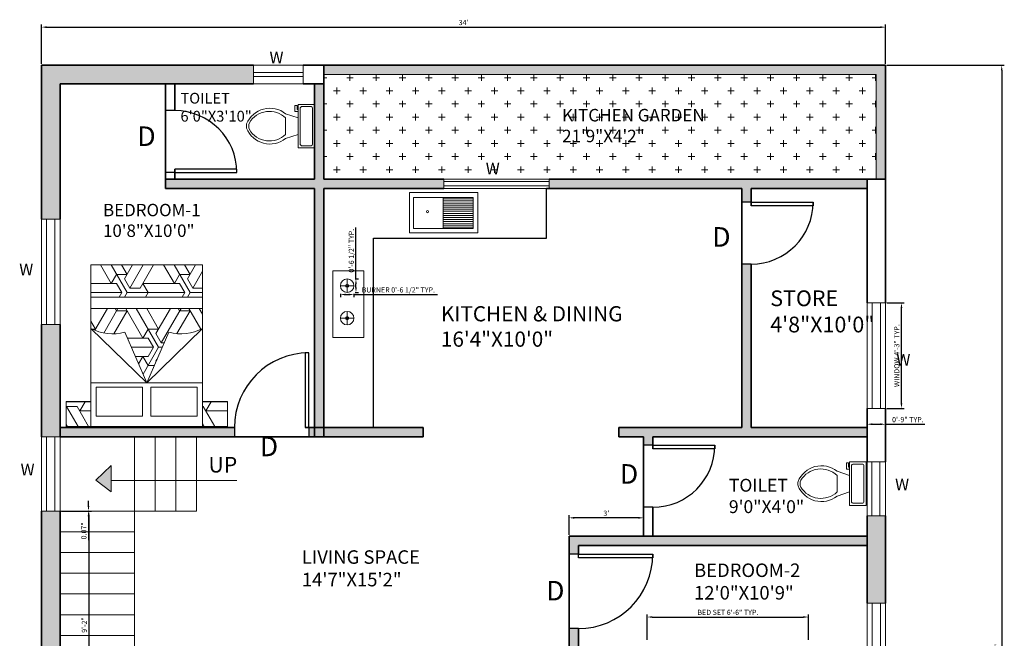
# Model space of a CAD drawing. Units: inches. Extents: x 1878 to 2382, y 1889 to 2524.
# Tile 2 of 2: x 1906 to 2382, y 2225 to 2524. Entities that reach past the tile are written whole.
import ezdxf

# ---------------------------------------------------------------- set-up
doc = ezdxf.new("R2010")
doc.units = ezdxf.units.IN
for name, color, linetype, lineweight in [('A-ANNO-DIMS', 2, 'Continuous', 18), ('A-ANNO-SYMB', 7, 'Continuous', 18), ('A-ANNO-TEXT', 7, 'Continuous', 18), ('A-AREA-IDEN', 7, 'Continuous', 18), ('A-DOOR', 4, 'Continuous', 25), ('A-EQPM', 8, 'Continuous', 18), ('A-FLOR-CASE', 8, 'Continuous', 25), ('A-FLOR-FIXT', 8, 'Continuous', 18), ('A-FLOR-FIXT-PATT', 8, 'Continuous', 13), ('A-FLOR-STRS', 7, 'Continuous', 18), ('A-FURN', 8, 'Continuous', 18), ('A-FURN-PATT', 252, 'Continuous', 13), ('A-WALL', 7, 'Continuous', 35), ('A-WALL-PATT', 251, 'Continuous', 13), ('L-PLNT', 3, 'Continuous', 18), ('L-PLNT-PATT', 3, 'Continuous', 13), ('windows', 5, 'Continuous', 18)]:
    doc.layers.add(name, color=color, linetype=linetype, lineweight=lineweight)
doc.styles.get("Standard").update_dxf_attribs({"font": 'arial.ttf'})
doc.dimstyles.new('ISO-25', dxfattribs={"dimtxt": 2.5, "dimasz": 2.5, "dimexe": 1.25, "dimexo": 0.625, "dimtad": 1, "dimlunit": 3, "dimtxsty": 'Standard', "dimcen": 2.5, "dimadec": 0, "dimazin": 0, "dimtfac": 1, "dimtmove": 0, "dimatfit": 3, "dimfxl": 1, "dimarcsym": 0})

# ---------------------------------------------------------------- blocks, each defined once
blk = doc.blocks.new('*U2')
for p, q in [((0, 0), (0, -4)), ((36, 0), (36, -4))]:
    blk.add_line(p, q)
blk.add_lwpolyline([(0, 0), (0, 36), (1.75, 36), (1.75, 0)], close=True)
blk.add_arc((0, 0), 36, 0, 90)
blk = doc.blocks.new('*U4')
for p, q in [((0, 0), (0, -4)), ((30, 0), (30, -4))]:
    blk.add_line(p, q)
blk.add_lwpolyline([(0, 0), (0, 30), (1.75, 30), (1.75, 0)], close=True)
blk.add_arc((0, 0), 30, 0, 90)
blk = doc.blocks.new('*U3')
for p, q in [((0, 0), (0, -4)), ((30, 0), (30, -4))]:
    blk.add_line(p, q)
blk.add_lwpolyline([(0, 0), (0, 30), (1.75, 30), (1.75, 0)], close=True)
blk.add_arc((0, 0), 30, 0, 90)
blk = doc.blocks.new('*U5')
for p, q in [((-30, 0), (-30, -4)), ((0, 0), (0, -4))]:
    blk.add_line(p, q)
blk.add_lwpolyline([(0, 0), (0, 30), (-1.75, 30), (-1.75, 0)], close=True)
blk.add_arc((0, 0), 30, 90, 180)
blk = doc.blocks.new('*U6')
for p, q in [((0, 0), (0, -4)), ((-36, 0), (-36, -4))]:
    blk.add_line(p, q)
blk.add_lwpolyline([(0, 0), (0, 36), (-1.75, 36), (-1.75, 0)], close=True)
blk.add_arc((0, 0), 36, 90, 180)
blk = doc.blocks.new('*U8')
for p, q in [((9.5, -6), (9.5, -2)), ((-10, -8.5), (-8, -8.5)), ((-10, -9.5), (-10, -8.5)), ((-7, -9.5), (-10, -9.5)), ((-8, -8.5), (-8, -8)), ((-7, -8), (-7, -9.5)), ((-4, -8), (-6, -14)), ((4, -8), (6, -14)), ((4, -14), (-4, -14))]:
    blk.add_line(p, q)
blk.add_lwpolyline([(10.5, -8), (10.5, 0), (-10.5, 0), (-10.5, -8)], close=True)
for points in [[(-9.5, -2), (-9.5, -6)], [(8.5, -1), (-8.5, -1)], [(-8.5, -7), (8.5, -7)]]:
    blk.add_lwpolyline(points)
for centre, radius, start, end in [((-8.62, -1.88), 0.884, 81.8699, 188.1301), ((8.62, -1.88), 0.884, 351.8699, 98.1301), ((-8.62, -6.12), 0.884, 171.8699, 278.1301), ((8.62, -6.12), 0.884, 261.8699, 8.1301), ((3.52, -21.58), 12.17, 141.4691, 247.9714), ((4.2, -21.82), 11.33, 136.3677, 238.9468), ((-3.52, -21.58), 12.17, 292.0284, 38.5307), ((-4.2, -21.82), 11.33, 301.053, 43.6321), ((0, -27.88), 4, 245.7318, 294.2682), ((0, -29), 4, 254.8605, 285.1395)]:
    blk.add_arc(centre, radius, start, end)
blk = doc.blocks.new('*D9')
at = {"layer": 'A-ANNO-DIMS', "color": 0, "lineweight": -2, "transparency": 16777216}
for p, q in [((1925.87, 2286.07), (1940.42, 2286.07)), ((1939.17, 2283.57), (1939.17, 2178.57)), ((1925.87, 2176.07), (1940.42, 2176.07))]:
    blk.add_line(p, q, dxfattribs=at)
at = {"layer": 'A-ANNO-DIMS', "color": 0, "transparency": 16777216}
for points in [[(1938.75, 2283.57), (1939.59, 2283.57), (1939.17, 2286.07)], [(1938.75, 2178.57), (1939.59, 2178.57), (1939.17, 2176.07)]]:
    blk.add_solid(points, dxfattribs=at)
at = {"layer": 'Defpoints', "color": 0, "transparency": 16777216}
for p in [(1925.24, 2286.07), (1925.24, 2176.07), (1939.17, 2176.07)]:
    blk.add_point(p, dxfattribs=at)
at = {"layer": 'A-ANNO-DIMS', "color": 0, "transparency": 16777216, "insert": (1937.27, 2231.07), "char_height": 2.5, "attachment_point": 5, "rotation": 90}
blk.add_mtext('9\'-2"', dxfattribs=at)
blk = doc.blocks.new('*D10')
at = {"layer": 'A-ANNO-DIMS', "color": 0, "lineweight": -2, "transparency": 16777216}
for p, q in [((1938.96, 2288.64), (1938.96, 2291.14)), ((1925.87, 2286.14), (1940.21, 2286.14)), ((1925.87, 2286.07), (1940.21, 2286.07)), ((1938.96, 2286.14), (1938.96, 2286.07)), ((1938.96, 2283.57), (1938.96, 2272.09))]:
    blk.add_line(p, q, dxfattribs=at)
at = {"layer": 'A-ANNO-DIMS', "color": 0, "transparency": 16777216}
for points in [[(1938.55, 2288.64), (1939.38, 2288.64), (1938.96, 2286.14)], [(1938.55, 2283.57), (1939.38, 2283.57), (1938.96, 2286.07)]]:
    blk.add_solid(points, dxfattribs=at)
at = {"layer": 'Defpoints', "color": 0, "transparency": 16777216}
for p in [(1925.24, 2286.14), (1925.24, 2286.07), (1938.96, 2286.07)]:
    blk.add_point(p, dxfattribs=at)
at = {"layer": 'A-ANNO-DIMS', "color": 0, "transparency": 16777216, "insert": (1937.06, 2276.58), "char_height": 2.5, "attachment_point": 5, "rotation": 90}
blk.add_mtext('0.07"', dxfattribs=at)
blk = doc.blocks.new('*D13')
at = {"layer": 'A-ANNO-DIMS', "color": 0, "lineweight": -2, "transparency": 16777216}
for p, q in [((2171.24, 2274.69), (2171.24, 2284.12)), ((2204.74, 2282.87), (2173.74, 2282.87)), ((2207.24, 2274.69), (2207.24, 2284.12))]:
    blk.add_line(p, q, dxfattribs=at)
at = {"layer": 'A-ANNO-DIMS', "color": 0, "transparency": 16777216}
for points in [[(2173.74, 2283.29), (2173.74, 2282.45), (2171.24, 2282.87)], [(2204.74, 2283.29), (2204.74, 2282.45), (2207.24, 2282.87)]]:
    blk.add_solid(points, dxfattribs=at)
at = {"layer": 'Defpoints', "color": 0, "transparency": 16777216}
for p in [(2171.24, 2282.87), (2171.24, 2274.07), (2207.24, 2274.07)]:
    blk.add_point(p, dxfattribs=at)
at = {"layer": 'A-ANNO-DIMS', "color": 0, "transparency": 16777216, "insert": (2189.24, 2284.77), "char_height": 2.5, "attachment_point": 5}
blk.add_mtext("3'", dxfattribs=at)
blk = doc.blocks.new('*D14')
at = {"layer": 'A-ANNO-DIMS', "color": 0, "lineweight": -2, "transparency": 16777216}
for p, q in [((1916.24, 2502.19), (1916.24, 2521.22)), ((1918.74, 2519.97), (2321.74, 2519.97)), ((2324.24, 2502.19), (2324.24, 2521.22))]:
    blk.add_line(p, q, dxfattribs=at)
at = {"layer": 'A-ANNO-DIMS', "color": 0, "transparency": 16777216}
for points in [[(1918.74, 2520.39), (1918.74, 2519.55), (1916.24, 2519.97)], [(2321.74, 2520.39), (2321.74, 2519.55), (2324.24, 2519.97)]]:
    blk.add_solid(points, dxfattribs=at)
at = {"layer": 'Defpoints', "color": 0, "transparency": 16777216}
for p in [(2324.24, 2519.97), (1916.24, 2501.57), (2324.24, 2501.57)]:
    blk.add_point(p, dxfattribs=at)
at = {"layer": 'A-ANNO-DIMS', "color": 0, "transparency": 16777216, "insert": (2120.24, 2521.87), "char_height": 2.5, "attachment_point": 5}
blk.add_mtext("34'", dxfattribs=at)
blk = doc.blocks.new('*D15')
at = {"layer": 'A-ANNO-DIMS', "color": 0, "lineweight": -2, "transparency": 16777216}
for p, q in [((2324.87, 2501.57), (2381.6, 2501.57)), ((2380.35, 2499.07), (2380.35, 1940.07)), ((2324.87, 1937.57), (2381.6, 1937.57))]:
    blk.add_line(p, q, dxfattribs=at)
at = {"layer": 'A-ANNO-DIMS', "color": 0, "transparency": 16777216}
for points in [[(2379.94, 2499.07), (2380.77, 2499.07), (2380.35, 2501.57)], [(2379.94, 1940.07), (2380.77, 1940.07), (2380.35, 1937.57)]]:
    blk.add_solid(points, dxfattribs=at)
at = {"layer": 'Defpoints', "color": 0, "transparency": 16777216}
for p in [(2324.24, 2501.57), (2324.24, 1937.57), (2380.35, 1937.57)]:
    blk.add_point(p, dxfattribs=at)
at = {"layer": 'A-ANNO-DIMS', "color": 0, "transparency": 16777216, "insert": (2378.48, 2219.57), "char_height": 2.5, "attachment_point": 5, "rotation": 90}
blk.add_mtext("47'", dxfattribs=at)
blk = doc.blocks.new('BED-DOUBLE-WITH-NIGHTSTANDS')
for p, q in [((39, 21.08), (12, 47.35)), ((39, 21.08), (28.35, 45.54)), ((39, 21.08), (66, 47.35)), ((39, 21.08), (49.65, 45.54)), ((66, 21.08), (12, 21.08)), ((36.92, 4.84), (36.92, 18.87)), ((40.92, 4.84), (40.92, 18.87)), ((0, 0), (0, 12)), ((0, 12), (12, 12)), ((78, 12), (66, 12)), ((78, 12), (78, 0)), ((12, 0), (0, 0)), ((66, 0), (78, 0))]:
    blk.add_line(p, q)
for points in [[(66, 78), (12, 78), (12, 0), (66, 0)], [(66, 56.97), (12, 56.97), (12, 62.38), (66, 62.38)]]:
    blk.add_lwpolyline(points, close=True)
for points in [[(36.92, 4.84), (14.54, 4.84), (14.54, 18.87), (36.92, 18.87)], [(40.92, 18.87), (63.29, 18.87), (63.29, 4.84), (40.92, 4.84)]]:
    blk.add_lwpolyline(points)
for centre, start, end in [((22.35, 66.17), 241.1931, 286.2111), ((55.65, 66.17), 253.7889, 298.8069)]:
    blk.add_arc(centre, 21.48, start, end)
blk = doc.blocks.new('WIN-51IN')
for p, q in [((4.5, 51), (0, 51)), ((0, 51), (9, 51)), ((0, 0), (0, 51)), ((2.5, 0), (2.5, 51)), ((6.5, 0), (6.5, 51)), ((9, 51), (9, 0)), ((0, 0), (9, 0)), ((9, 0), (4.5, 0))]:
    blk.add_line(p, q)
blk = doc.blocks.new('COOKTOP-BURNER')
for p, q in [((3.27, 6.54), (3.27, 0)), ((0, 3.27), (6.54, 3.27))]:
    blk.add_line(p, q)
for radius in [3.27, 0.76]:
    blk.add_circle((3.27, 3.27), radius)
blk = doc.blocks.new('*D21')
at = {"layer": 'A-ANNO-DIMS', "color": 0, "lineweight": -2, "transparency": 16777216}
for p, q in [((2209, 2223.87), (2209, 2236.19)), ((2211.5, 2234.94), (2284.5, 2234.94)), ((2287, 2223.87), (2287, 2236.19))]:
    blk.add_line(p, q, dxfattribs=at)
at = {"layer": 'A-ANNO-DIMS', "color": 0, "transparency": 16777216}
for points in [[(2211.5, 2235.36), (2211.5, 2234.53), (2209, 2234.94)], [(2284.5, 2235.36), (2284.5, 2234.53), (2287, 2234.94)]]:
    blk.add_solid(points, dxfattribs=at)
at = {"layer": 'Defpoints', "color": 0, "transparency": 16777216}
for p in [(2287, 2234.94), (2209, 2223.24), (2287, 2223.24)]:
    blk.add_point(p, dxfattribs=at)
at = {"layer": 'A-ANNO-DIMS', "color": 0, "transparency": 16777216, "insert": (2248, 2236.86), "char_height": 2.5, "attachment_point": 5}
blk.add_mtext('BED SET 6\'-6" TYP.', dxfattribs=at)
blk = doc.blocks.new('*D23')
at = {"layer": 'A-ANNO-DIMS', "color": 0, "lineweight": -2, "transparency": 16777216}
for p, q in [((2324.87, 2386.74), (2333.14, 2386.74)), ((2331.89, 2338.24), (2331.89, 2384.24)), ((2324.87, 2335.74), (2333.14, 2335.74))]:
    blk.add_line(p, q, dxfattribs=at)
at = {"layer": 'A-ANNO-DIMS', "color": 0, "transparency": 16777216}
for points in [[(2331.47, 2384.24), (2332.31, 2384.24), (2331.89, 2386.74)], [(2331.47, 2338.24), (2332.31, 2338.24), (2331.89, 2335.74)]]:
    blk.add_solid(points, dxfattribs=at)
at = {"layer": 'Defpoints', "color": 0, "transparency": 16777216}
for p in [(2324.24, 2386.74), (2331.89, 2386.74), (2324.24, 2335.74)]:
    blk.add_point(p, dxfattribs=at)
at = {"layer": 'A-ANNO-DIMS', "color": 0, "transparency": 16777216, "insert": (2329.97, 2361.24), "char_height": 2.5, "attachment_point": 5, "rotation": 90}
blk.add_mtext('WINDOW 4\'-3" TYP.', dxfattribs=at)
blk = doc.blocks.new('*D24')
at = {"layer": 'A-ANNO-DIMS', "color": 0, "lineweight": -2, "transparency": 16777216}
for p, q in [((2315.24, 2335.12), (2315.24, 2326.84)), ((2324.24, 2335.12), (2324.24, 2326.84)), ((2317.74, 2328.09), (2321.74, 2328.09)), ((2324.24, 2328.09), (2343.23, 2328.09))]:
    blk.add_line(p, q, dxfattribs=at)
at = {"layer": 'A-ANNO-DIMS', "color": 0, "transparency": 16777216}
for points in [[(2317.74, 2328.51), (2317.74, 2327.68), (2315.24, 2328.09)], [(2321.74, 2328.51), (2321.74, 2327.68), (2324.24, 2328.09)]]:
    blk.add_solid(points, dxfattribs=at)
at = {"layer": 'Defpoints', "color": 0, "transparency": 16777216}
for p in [(2315.24, 2335.74), (2324.24, 2335.74), (2324.24, 2328.09)]:
    blk.add_point(p, dxfattribs=at)
at = {"layer": 'A-ANNO-DIMS', "color": 0, "transparency": 16777216, "insert": (2334.99, 2330), "char_height": 2.5, "attachment_point": 5}
blk.add_mtext('0\'-9" TYP.', dxfattribs=at)
blk = doc.blocks.new('*D25')
at = {"layer": 'A-ANNO-DIMS', "color": 0, "lineweight": -2, "transparency": 16777216}
for p, q in [((2060.72, 2391.12), (2060.72, 2389.51)), ((2063.22, 2390.76), (2064.76, 2390.76)), ((2067.26, 2391.12), (2067.26, 2389.51)), ((2067.26, 2390.76), (2107.68, 2390.76))]:
    blk.add_line(p, q, dxfattribs=at)
at = {"layer": 'A-ANNO-DIMS', "color": 0, "transparency": 16777216}
for points in [[(2063.22, 2391.18), (2063.22, 2390.34), (2060.72, 2390.76)], [(2064.76, 2391.18), (2064.76, 2390.34), (2067.26, 2390.76)]]:
    blk.add_solid(points, dxfattribs=at)
at = {"layer": 'Defpoints', "color": 0, "transparency": 16777216}
for p in [(2060.72, 2391.74), (2067.26, 2391.74), (2067.26, 2390.76)]:
    blk.add_point(p, dxfattribs=at)
at = {"layer": 'A-ANNO-DIMS', "color": 0, "transparency": 16777216, "insert": (2088.72, 2392.68), "char_height": 2.5, "attachment_point": 5}
blk.add_mtext('BURNER 0\'-6 1/2" TYP.', dxfattribs=at)
blk = doc.blocks.new('*D26')
at = {"layer": 'A-ANNO-DIMS', "color": 0, "lineweight": -2, "transparency": 16777216}
for p, q in [((2068.24, 2398.28), (2068.24, 2423.09)), ((2067.88, 2398.28), (2069.49, 2398.28)), ((2068.24, 2394.24), (2068.24, 2395.78)), ((2067.88, 2391.74), (2069.49, 2391.74))]:
    blk.add_line(p, q, dxfattribs=at)
at = {"layer": 'A-ANNO-DIMS', "color": 0, "transparency": 16777216}
for points in [[(2067.82, 2395.78), (2068.66, 2395.78), (2068.24, 2398.28)], [(2067.82, 2394.24), (2068.66, 2394.24), (2068.24, 2391.74)]]:
    blk.add_solid(points, dxfattribs=at)
at = {"layer": 'Defpoints', "color": 0, "transparency": 16777216}
for p in [(2067.26, 2398.28), (2068.24, 2398.28), (2067.26, 2391.74)]:
    blk.add_point(p, dxfattribs=at)
at = {"layer": 'A-ANNO-DIMS', "color": 0, "transparency": 16777216, "insert": (2066.32, 2411.94), "char_height": 2.5, "attachment_point": 5, "rotation": 90}
blk.add_mtext('0\'-6 1/2" TYP.', dxfattribs=at)

msp = doc.modelspace()

# ---------------------------------------------------------------- hatches: boundary and pattern name
at = {"layer": 'A-ANNO-SYMB'}
h = msp.add_hatch(color=256, dxfattribs=at)
h.dxf.hatch_style = 1
h.paths.add_polyline_path([(1949.873, 2308.099), (1942.575, 2300.99), (1949.873, 2295.451)])
at = {"layer": 'A-FLOR-FIXT-PATT'}
h = msp.add_hatch(dxfattribs=at)
h.set_pattern_fill('ANSI31', color=256, scale=0.3149606, angle=-45, style=0)
h.paths.add_polyline_path([(2110.458, 2422.666), (2124.915, 2422.666), (2124.915, 2437.672), (2110.458, 2437.672)])
at = {"layer": 'A-FURN-PATT'}
h = msp.add_hatch(dxfattribs=at)
h.set_pattern_fill('ESCHER', color=256, angle=180)
h.set_pattern_definition([(240, (4365.518, 4820.139), (30.48, 7e-09), [27.94, -2.54]), (360, (4365.518, 4820.139), (-15.24, 26.39645), [27.94, -2.54]), (120, (4365.518, 4820.139), (-30.48, 7e-09), [27.94, -2.54]), (240, (4362.978, 4820.139), (30.48, 7e-09), [5.08, -25.4]), (120, (4362.978, 4820.139), (-30.48, 7e-09), [5.08, -25.4]), (240, (4366.788, 4817.94), (30.48, 7e-09), [5.08, -25.4]), (360, (4366.788, 4817.94), (-15.24, 26.39645), [5.08, -25.4]), (120, (4366.788, 4822.338), (-30.48, 7e-09), [5.08, -25.4]), (360, (4366.788, 4822.338), (-15.24, 26.39645), [5.08, -25.4]), (240, (4375.678, 4820.139), (30.48, 7e-09), [5.08, -25.4]), (120, (4375.678, 4820.139), (-30.48, 7e-09), [5.08, -25.4]), (240, (4360.438, 4828.937), (30.48, 7e-09), [5.08, -25.4]), (360, (4360.438, 4828.937), (-15.24, 26.39645), [5.08, -25.4]), (120, (4360.438, 4811.34), (-30.48, 7e-09), [5.08, -25.4]), (360, (4360.438, 4811.34), (-15.24, 26.39645), [5.08, -25.4]), (180, (4360.438, 4815.74), (15.24, -26.39645), [17.78, -12.7]), (180, (4360.438, 4824.538), (15.24, -26.39645), [17.78, -12.7]), (300, (4364.248, 4813.54), (30.48, -7e-09), [17.78, -12.7]), (300, (4371.868, 4817.94), (30.48, -7e-09), [17.78, -12.7]), (60, (4371.868, 4822.338), (-15.24, 26.39645), [17.78, -12.7]), (60, (4364.248, 4826.738), (-15.24, 26.39645), [17.78, -12.7])])
h.paths.add_polyline_path([(1967.133, 2348.159), (1977.782, 2372.62, 0.1989938), (1994.133, 2374.424), (1994.133, 2384.048), (1940.133, 2384.048), (1940.133, 2374.424, 0.1989938), (1956.484, 2372.62)])
h.paths.add_polyline_path([(1994.133, 2389.462), (1994.133, 2405.079), (1940.133, 2405.079), (1940.133, 2389.462)])
h.paths.add_polyline_path([(1928.133, 2339.079), (1928.133, 2327.079), (1940.133, 2327.079), (1940.133, 2339.079)])
h.paths.add_polyline_path([(2006.133, 2339.079), (1994.133, 2339.079), (1994.133, 2327.079), (2006.133, 2327.079)])
at = {"layer": 'A-WALL-PATT'}
h = msp.add_hatch(color=256, dxfattribs=at)
h.dxf.hatch_style = 1
h.paths.add_polyline_path([(1925.241, 2376.261), (1916.241, 2376.261), (1916.241, 2322.068), (1920.741, 2322.068), (1925.241, 2322.068)])
h.paths.add_polyline_path([(1925.241, 2286.14), (1916.241, 2286.068), (1916.241, 2097.507), (1920.741, 2097.507), (1925.241, 2097.507)])
h.paths.add_polyline_path([(1925.241, 2046.507), (1916.241, 2046.507), (1916.241, 1993.068), (1925.241, 1993.068), (2100.229, 1993.068), (2100.229, 1997.568), (2100.229, 2002.068), (2052.741, 2002.068), (2052.741, 2135.568), (2048.241, 2135.568), (2048.241, 2002.068), (1925.241, 2002.068)])
h.paths.add_polyline_path([(2175.741, 2006.935), (2175.253, 2006.935), (2171.241, 2006.935), (2171.241, 2002.068), (2136.229, 2002.068), (2136.229, 1993.068), (2171.241, 1993.068), (2175.741, 1993.068)])
h.paths.add_polyline_path([(1925.241, 2492.568), (2018.709, 2492.568), (2018.709, 2497.068), (2018.709, 2501.568), (1916.241, 2501.568), (1916.241, 2427.261), (1925.241, 2427.261)])
h.paths.add_polyline_path([(2324.241, 2501.568), (2052.741, 2501.568), (2052.741, 2497.068), (2319.741, 2497.068), (2319.741, 2446.568), (2324.241, 2446.568)])
h.paths.add_polyline_path([(2110.638, 2446.568), (2052.741, 2446.568), (2052.741, 2492.568), (2048.241, 2492.568), (2048.241, 2446.568), (1976.241, 2446.568), (1976.241, 2442.068), (2048.241, 2442.068), (2048.241, 2326.568), (2052.741, 2326.568), (2052.741, 2442.068), (2110.638, 2442.068), (2110.638, 2444.318)])
h.paths.add_polyline_path([(2100.741, 2326.568), (2052.741, 2326.568), (2052.741, 2322.068), (2100.741, 2322.068)])
h.paths.add_polyline_path([(2052.741, 2326.568), (2048.241, 2326.568), (2048.241, 2322.068), (2052.741, 2322.068)])
h.paths.add_polyline_path([(2048.241, 2326.568), (2045.469, 2326.568), (2045.469, 2326.565), (2045.469, 2322.565), (2045.469, 2322.068), (2048.241, 2322.068)])
h.paths.add_polyline_path([(2009.469, 2326.568), (1925.241, 2326.568), (1925.241, 2322.068), (2009.469, 2322.068), (2009.469, 2322.565)])
h.paths.add_polyline_path([(2315.241, 2326.568), (2259.241, 2326.568), (2259.241, 2405.456), (2255.232, 2405.456), (2254.741, 2405.456), (2254.741, 2326.568), (2207.241, 2326.568), (2195.241, 2326.568), (2195.241, 2322.068), (2207.241, 2322.068), (2207.241, 2317.983), (2207.736, 2317.983), (2211.741, 2317.983), (2211.741, 2322.068), (2315.241, 2322.068)])
h.paths.add_polyline_path([(2315.241, 2446.568), (2161.638, 2446.568), (2161.638, 2442.068), (2254.741, 2442.068), (2254.741, 2435.456), (2255.232, 2435.456), (2259.241, 2435.456), (2259.241, 2442.068), (2315.241, 2442.068)])
h.paths.add_polyline_path([(2315.241, 2274.068), (2207.241, 2274.068), (2171.241, 2274.068), (2171.241, 2265.326), (2171.731, 2265.326), (2175.741, 2265.326), (2175.741, 2269.568), (2315.241, 2269.568)])
h.paths.add_polyline_path([(2226.778, 2011.849), (2261.831, 2011.849), (2261.831, 2029.017), (2226.778, 2029.017)], flags=9)
h.paths.add_polyline_path([(2187.32, 2282.174), (2191.18, 2282.174), (2191.18, 2287.326), (2187.32, 2287.326)], flags=9)
h.paths.add_polyline_path([(2140.304, 2010.813), (2177.357, 2010.813), (2177.357, 2025.4), (2140.304, 2025.4)], flags=9)
h.paths.add_polyline_path([(2106.343, 2361.376), (2203.937, 2361.376), (2203.937, 2388.801), (2106.343, 2388.801)], flags=9)
h.paths.add_polyline_path([(2229.025, 2239.686), (2287.846, 2239.686), (2287.846, 2264.045), (2229.025, 2264.045)], flags=9)
h.paths.add_polyline_path([(2039.47, 2246.058), (2106.461, 2246.058), (2106.461, 2270.435), (2039.47, 2270.435)], flags=9)
h.paths.add_polyline_path([(2080.264, 2072.343), (2149.799, 2072.343), (2149.799, 2093.991), (2080.264, 2093.991)], flags=9)
h = msp.add_hatch(color=256, dxfattribs=at)
h.dxf.hatch_style = 1
h.paths.add_polyline_path([(2324.241, 2283.876), (2315.241, 2283.876), (2315.241, 2241.596), (2324.241, 2241.596)])
h.paths.add_polyline_path([(2324.241, 2190.596), (2315.241, 2190.596), (2315.241, 1946.568), (2315.241, 1937.568), (2324.241, 1937.568)])
h.paths.add_polyline_path([(2315.241, 2145.068), (2175.741, 2145.068), (2175.741, 2229.326), (2171.731, 2229.326), (2171.241, 2229.326), (2171.241, 2145.068), (2171.241, 2140.568), (2171.241, 2140.068), (2160.741, 2140.068), (2160.741, 2135.568), (2171.241, 2135.568), (2171.241, 2042.935), (2175.253, 2042.935), (2175.741, 2042.935), (2175.741, 2140.068), (2315.241, 2140.068)])
at = {"layer": 'L-PLNT-PATT'}
h = msp.add_hatch(dxfattribs=at)
h.set_pattern_fill('CROSS', color=256)
h.paths.add_polyline_path([(2319.741, 2497.068), (2052.741, 2497.068), (2052.741, 2492.568), (2052.741, 2446.568), (2315.241, 2446.568), (2319.741, 2446.568)])

# ---------------------------------------------------------------- linework, layer by layer
at = {"layer": 'A-ANNO-SYMB'}
for p, q in [((1949.873, 2308.099), (1942.575, 2300.99)), ((1949.873, 2295.451), (1949.873, 2308.099)), ((1942.575, 2300.99), (1949.873, 2295.451)), ((2010.617, 2300.952), (1949.873, 2300.952)), ((1949.873, 2300.952), (1949.873, 2295.451))]:
    msp.add_line(p, q, dxfattribs=at)
at = {"layer": 'A-DOOR'}
for p, q in [((1976.689, 2479.666), (1976.241, 2479.666)), ((1976.689, 2479.666), (1976.689, 2479.666)), ((1976.689, 2449.666), (1976.241, 2449.666)), ((2255.232, 2435.456), (2254.741, 2435.456)), ((2255.232, 2405.456), (2254.741, 2405.456)), ((2009.469, 2322.565), (2009.469, 2322.068)), ((2045.469, 2322.565), (2045.469, 2322.068)), ((2207.736, 2317.983), (2207.241, 2317.983)), ((2207.736, 2287.983), (2207.241, 2287.983)), ((2171.731, 2265.326), (2171.241, 2265.326)), ((2171.731, 2229.326), (2171.241, 2229.326))]:
    msp.add_line(p, q, dxfattribs=at)
at = {"layer": 'A-EQPM'}
msp.add_lwpolyline([(2057.035, 2402.205), (2072.05, 2402.205), (2072.05, 2370.086), (2057.035, 2370.086)], close=True, dxfattribs=at)
at = {"layer": 'A-FLOR-CASE'}
for p, q in [((2160.349, 2418.068), (2160.349, 2442.068)), ((2076.741, 2326.568), (2076.741, 2418.068)), ((2076.741, 2418.068), (2160.349, 2418.068))]:
    msp.add_line(p, q, dxfattribs=at)
at = {"layer": 'A-FLOR-FIXT'}
msp.add_line((2110.458, 2437.672), (2110.458, 2422.666), dxfattribs=at)
for points in [[(2094.139, 2440.028), (2127.149, 2440.028), (2127.149, 2420.558), (2094.139, 2420.558)], [(2096.001, 2437.672), (2124.915, 2437.672), (2124.915, 2422.666), (2096.001, 2422.666)]]:
    msp.add_lwpolyline(points, close=True, dxfattribs=at)
msp.add_circle((2102.839, 2430.858), 0.534, dxfattribs=at)
at = {"layer": 'A-FLOR-STRS'}
for p, q in [((1961.241, 2286.068), (1961.241, 2322.068)), ((1971.241, 2286.068), (1971.241, 2322.068)), ((1981.241, 2286.068), (1981.241, 2322.068)), ((1991.241, 2286.068), (1991.241, 2322.068)), ((1925.241, 2286.068), (1925.241, 2176.068)), ((1925.241, 2286.068), (1961.241, 2286.068)), ((1961.241, 2286.068), (1961.241, 2276.068)), ((1961.241, 2286.068), (1991.241, 2286.068)), ((1961.241, 2276.068), (1925.241, 2276.068)), ((1961.241, 2276.068), (1961.241, 2176.068)), ((1961.241, 2266.068), (1925.241, 2266.068)), ((1961.241, 2256.068), (1925.241, 2256.068)), ((1961.241, 2246.068), (1925.241, 2246.068)), ((1961.241, 2236.068), (1925.241, 2236.068)), ((1961.241, 2226.068), (1925.241, 2226.068))]:
    msp.add_line(p, q, dxfattribs=at)
at = {"layer": 'A-WALL'}
for p, q in [((1916.241, 2501.568), (2018.709, 2501.568)), ((1916.241, 2427.261), (1916.241, 2501.568)), ((2042.709, 2501.568), (2324.241, 2501.568)), ((2052.741, 2492.568), (2052.741, 2501.568)), ((2324.241, 2501.568), (2324.241, 2386.744)), ((1925.241, 2492.568), (2018.709, 2492.568)), ((1925.241, 2427.261), (1925.241, 2492.568)), ((1976.241, 2442.068), (1976.241, 2492.568)), ((1980.741, 2479.666), (1980.741, 2492.568)), ((2042.709, 2492.568), (2052.741, 2492.568)), ((2048.241, 2446.568), (2048.241, 2492.568)), ((2052.741, 2446.568), (2052.741, 2492.568)), ((1980.741, 2446.568), (1980.741, 2451.416)), ((1976.241, 2446.568), (2048.241, 2446.568)), ((2052.741, 2446.568), (2110.638, 2446.568)), ((2161.638, 2446.568), (2315.241, 2446.568)), ((2315.241, 2446.568), (2315.241, 2386.744)), ((2315.241, 2446.568), (2324.241, 2446.568)), ((1976.241, 2442.068), (2048.241, 2442.068)), ((2048.241, 2322.068), (2048.241, 2442.068)), ((2052.741, 2322.068), (2052.741, 2442.068)), ((2052.741, 2442.068), (2110.638, 2442.068)), ((2160.349, 2442.068), (2254.741, 2442.068)), ((2254.741, 2442.068), (2254.741, 2326.568)), ((2259.241, 2442.068), (2259.241, 2433.706)), ((2259.241, 2442.068), (2315.241, 2442.068)), ((2259.241, 2405.456), (2259.241, 2326.568)), ((1916.241, 2322.068), (1916.241, 2376.261)), ((1925.241, 2322.068), (1925.241, 2376.261)), ((2315.241, 2335.744), (2315.241, 2309.876)), ((2324.241, 2335.744), (2324.241, 2309.876)), ((2009.469, 2326.568), (1925.241, 2326.568)), ((2052.741, 2326.568), (2043.719, 2326.568)), ((2052.741, 2326.568), (2100.741, 2326.568)), ((2100.741, 2326.568), (2100.741, 2322.068)), ((2195.241, 2322.068), (2195.241, 2326.568)), ((2195.241, 2326.568), (2207.241, 2326.568)), ((2254.741, 2326.568), (2207.241, 2326.568)), ((2259.241, 2326.568), (2315.241, 2326.568)), ((2052.741, 2322.068), (1925.241, 2322.068)), ((2100.741, 2322.068), (2052.741, 2322.068)), ((2207.241, 2322.068), (2195.241, 2322.068)), ((2207.241, 2322.068), (2207.241, 2274.068)), ((2207.241, 2322.068), (2207.241, 2318.068)), ((2315.241, 2322.068), (2211.741, 2322.068)), ((2211.741, 2322.068), (2211.741, 2316.233)), ((2254.741, 2322.068), (2315.241, 2322.068)), ((1916.241, 2097.507), (1916.241, 2286.068)), ((1925.241, 2286.14), (1925.241, 2286.068)), ((1925.241, 2097.507), (1925.241, 2286.14)), ((2211.741, 2287.983), (2211.741, 2274.068)), ((2315.241, 2283.876), (2315.241, 2241.596)), ((2324.241, 2283.876), (2324.241, 2241.596)), ((2207.241, 2274.068), (2171.241, 2274.068)), ((2171.241, 2274.068), (2171.241, 2269.568)), ((2171.241, 2145.068), (2171.241, 2274.068)), ((2315.241, 2274.068), (2207.241, 2274.068)), ((2175.741, 2269.568), (2315.241, 2269.568)), ((2175.741, 2265.326), (2175.741, 2269.568)), ((2175.741, 2145.068), (2175.741, 2229.326))]:
    msp.add_line(p, q, dxfattribs=at)
at = {"layer": 'L-PLNT'}
for p, q in [((2052.741, 2497.068), (2319.741, 2497.068)), ((2319.741, 2497.068), (2319.741, 2446.568))]:
    msp.add_line(p, q, dxfattribs=at)
at = {"layer": 'windows'}
for p, q in [((2018.709, 2501.568), (2018.709, 2492.568)), ((2018.709, 2501.568), (2042.709, 2501.568)), ((2042.709, 2497.068), (2042.709, 2501.568)), ((2042.709, 2501.568), (2042.709, 2492.568)), ((2018.709, 2498.068), (2042.709, 2498.068)), ((2018.709, 2492.568), (2018.709, 2497.068)), ((2018.709, 2496.068), (2042.709, 2496.068)), ((2042.709, 2492.568), (2018.709, 2492.568)), ((2110.638, 2446.568), (2110.638, 2442.068)), ((2161.638, 2446.568), (2110.638, 2446.568)), ((2161.638, 2444.318), (2161.638, 2446.568)), ((2161.638, 2446.568), (2161.638, 2442.068)), ((2110.638, 2445.318), (2161.638, 2445.318)), ((2110.638, 2442.068), (2110.638, 2444.318)), ((2110.638, 2443.318), (2161.638, 2443.318)), ((2161.638, 2442.068), (2110.638, 2442.068)), ((1920.741, 2427.261), (1916.241, 2427.261)), ((1916.241, 2427.261), (1925.241, 2427.261)), ((1916.241, 2427.261), (1916.241, 2376.261)), ((1918.741, 2376.261), (1918.741, 2427.261)), ((1922.741, 2376.261), (1922.741, 2427.261)), ((1925.241, 2427.261), (1925.241, 2376.261)), ((1925.241, 2376.261), (1916.241, 2376.261)), ((1916.241, 2376.261), (1920.741, 2376.261)), ((1925.241, 2322.068), (1916.241, 2322.068)), ((1916.241, 2322.068), (1920.741, 2322.068)), ((1916.241, 2322.068), (1916.241, 2286.068)), ((1918.741, 2322.068), (1918.741, 2286.14)), ((1922.741, 2322.068), (1922.741, 2286.14)), ((1925.241, 2322.068), (1925.241, 2286.14)), ((2314.768, 2309.876), (2324.241, 2309.876)), ((2315.241, 2283.876), (2315.241, 2309.876)), ((2317.505, 2307.876), (2317.505, 2309.876)), ((2324.241, 2309.876), (2319.505, 2309.876)), ((2321.505, 2307.876), (2321.505, 2309.876)), ((2324.241, 2309.876), (2324.241, 2283.876)), ((2317.505, 2307.876), (2317.505, 2283.876)), ((2321.505, 2307.876), (2321.505, 2283.876)), ((1925.241, 2286.14), (1916.241, 2286.068)), ((1920.741, 2286.14), (1925.241, 2286.14)), ((2319.505, 2283.876), (2315.241, 2283.876)), ((2315.241, 2283.876), (2324.241, 2283.876))]:
    msp.add_line(p, q, dxfattribs=at)

# ---------------------------------------------------------------- block references
at = {"layer": 'A-DOOR', "rotation": 270}
for name, p in [('*U5', (1980.689, 2449.666)), ('*U3', (2259.232, 2435.456)), ('*U4', (2211.736, 2317.983)), ('*U2', (2175.731, 2265.326))]:
    msp.add_blockref(name, p, dxfattribs=at)
at = {"layer": 'A-DOOR'}
msp.add_blockref('*U6', (2045.469, 2326.565), dxfattribs=at)
at = {"layer": 'A-EQPM'}
for p in [(2060.72, 2391.741), (2060.72, 2376.086)]:
    msp.add_blockref('COOKTOP-BURNER', p, dxfattribs=at)
at = {"layer": 'A-FLOR-FIXT', "rotation": 270}
for p in [(2048.261, 2472.14), (2314.768, 2299.376)]:
    msp.add_blockref('*U8', p, dxfattribs=at)
at = {"layer": 'A-FURN'}
msp.add_blockref('BED-DOUBLE-WITH-NIGHTSTANDS', (1928.133, 2327.079), dxfattribs=at)
at = {"layer": 'windows'}
msp.add_blockref('WIN-51IN', (2315.241, 2335.743), dxfattribs=at)
at = {"layer": 'windows', "extrusion": (0, 0, -1), "zscale": -1}
msp.add_blockref('WIN-51IN', (-2324.242, 2190.595), dxfattribs=at)

# ---------------------------------------------------------------- texts
at = {"layer": 'A-ANNO-TEXT', "attachment_point": 1}
for s, width, gutter_width, insert, char_height in [('W', 334.92413, 28.121, (2026.461, 2508.128), 5.624), ('D', 211.86968, 47.154, (1962.573, 2471.986), 9.431), ('W', 334.92413, 28.121, (2130.986, 2454.429), 5.624), ('D', 211.86968, 47.154, (2240.441, 2423.326), 9.431), ('W', 334.92413, 28.121, (1905.51, 2405.676), 5.624), ('W', 334.92413, 28.121, (2329.457, 2362.015), 5.624), ('D', 211.86968, 47.154, (2021.777, 2322.068), 9.431), ('W', 334.92413, 28.121, (1906.154, 2309.006), 5.624), ('UP', 63.8866, 37.641, (1996.94, 2312.302), 7.5281), ('D', 211.86968, 47.154, (2195.805, 2308.802), 9.431), ('W', 334.92413, 28.121, (2328.842, 2301.797), 5.624), ('D', 211.86968, 47.154, (2160.165, 2252.385), 9.431)]:
    msp.add_mtext_dynamic_manual_height_columns(s, width=width, gutter_width=gutter_width, heights=[0], dxfattribs=dict(at, insert=insert, char_height=char_height))
at = {"layer": 'A-AREA-IDEN', "attachment_point": 1}
for s, width, gutter_width, heights, insert, char_height in [('TOILET\\P6\'0"X3\'10"', 21.36598, 26.035, [0], (1983.408, 2488.234), 5.2071), ('KITCHEN GARDEN\\P21\'9"X4\'2"', 152.24218, 30.172, [0], (2167.874, 2480.46), 6.03443), ('BEDROOM-1\\P10\'8"X10\'0"', 112.45203, 29.973, [0], (1945.995, 2434.597), 5.99464), ('STORE\\P4\'8"X10\'0"', 127.23393, 38.034, [0], (2268.481, 2392.764), 7.6067), ('KITCHEN & DINING\\P16\'4"X10\'0"', 132.28599, 36.748, [0], (2109.298, 2385.143), 7.34952), ('TOILET\\P9\'0"X4\'0"', 62.32474, 31.051, [0], (2248.482, 2301.717), 6.2102), ('LIVING SPACE \\P14\'7"X15\'2"\\P ', 67.57238, 32.665, [28.447], (2042.097, 2267.184), 6.53292), ('BEDROOM-2\\P12\'0"X10\'9" ', 128.90971, 32.641, [0], (2231.65, 2260.801), 6.52814)]:
    msp.add_mtext_dynamic_manual_height_columns(s, width=width, gutter_width=gutter_width, heights=heights, dxfattribs=dict(at, insert=insert, char_height=char_height))

# ---------------------------------------------------------------- dimensions: what is measured, and where the dimension line sits
at = {"layer": 'A-ANNO-DIMS'}
for base, p1, p2, picture, middle in [((2324.241, 2519.97), (1916.241, 2501.568), (2324.241, 2501.568), '*D14', (2120.241, 2521.872)), ((2171.241, 2282.87), (2207.241, 2274.068), (2171.241, 2274.068), '*D13', (2189.241, 2284.772))]:
    dim = msp.add_linear_dim(base=base, p1=p1, p2=p2, dimstyle='ISO-25', override={"dimclrd": 0, "dimclre": 0, "dimclrt": 0}, dxfattribs=at)
    dim.commit()
    dim.dimension.update_dxf_attribs({"geometry": picture, "text_midpoint": middle})
for base, p1, p2, picture, middle in [((2380.352, 1937.568), (2324.241, 2501.568), (2324.241, 1937.568), '*D15', (2378.477, 2219.568)), ((1938.962, 2286.068), (1925.241, 2286.14), (1925.241, 2286.068), '*D10', (1937.061, 2276.579)), ((1939.171, 2176.068), (1925.241, 2286.068), (1925.241, 2176.068), '*D9', (1937.269, 2231.068))]:
    dim = msp.add_linear_dim(base=base, p1=p1, p2=p2, angle=90, dimstyle='ISO-25', override={"dimclrd": 0, "dimclre": 0, "dimclrt": 0}, dxfattribs=at)
    dim.commit()
    dim.dimension.update_dxf_attribs({"geometry": picture, "text_midpoint": middle})
for base, p1, p2, text, picture, middle in [((2068.239, 2398.278), (2067.258, 2391.741), (2067.258, 2398.278), '<> TYP.', '*D26', (2066.321, 2411.935)), ((2331.891, 2386.744), (2324.241, 2335.744), (2324.241, 2386.744), 'WINDOW <> TYP.', '*D23', (2329.972, 2361.244))]:
    dim = msp.add_linear_dim(base=base, p1=p1, p2=p2, angle=90, text=text, dimstyle='ISO-25', override={"dimdec": 1, "dimlfac": 1, "dimrnd": 0, "dimzin": 1, "dimdsep": 46, "dimlunit": 4, "dimfrac": 2}, dxfattribs=at)
    dim.commit()
    dim.dimension.update_dxf_attribs({"geometry": picture, "text_midpoint": middle})
for base, p1, p2, text, picture, middle in [((2067.258, 2390.76), (2060.72, 2391.741), (2067.258, 2391.741), 'BURNER <> TYP.', '*D25', (2088.719, 2392.678)), ((2324.241, 2328.094), (2315.241, 2335.744), (2324.241, 2335.744), '<> TYP.', '*D24', (2334.986, 2329.995)), ((2286.998, 2234.943), (2208.998, 2223.243), (2286.998, 2223.243), 'BED SET <> TYP.', '*D21', (2247.998, 2236.86))]:
    dim = msp.add_linear_dim(base=base, p1=p1, p2=p2, text=text, dimstyle='ISO-25', override={"dimdec": 1, "dimlfac": 1, "dimrnd": 0, "dimzin": 1, "dimdsep": 46, "dimlunit": 4, "dimfrac": 2}, dxfattribs=at)
    dim.commit()
    dim.dimension.update_dxf_attribs({"geometry": picture, "text_midpoint": middle})

doc.saveas('drawing.dxf')
